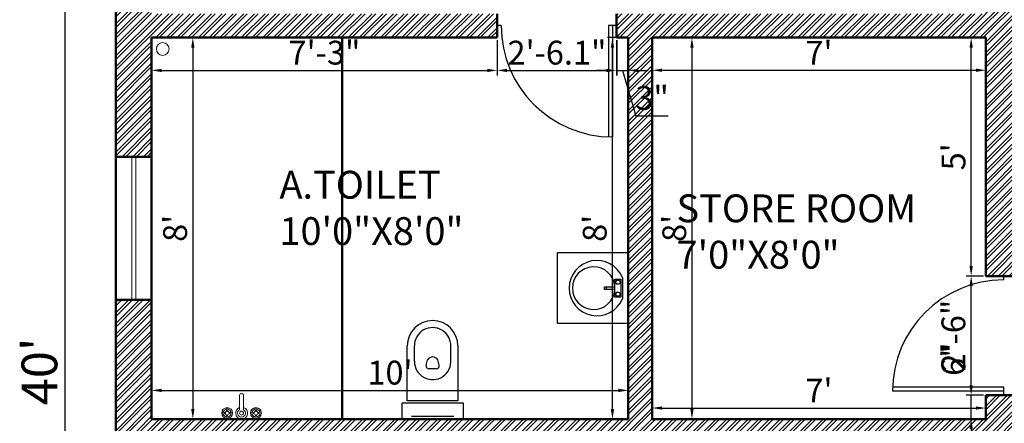
# Model space of a CAD drawing. Units: inches. Extents: x 3590 to 5167, y 65 to 1917.
# Tile 9 of 100: x 4396 to 4644, y 336 to 438. Entities that reach past the tile are written whole.
import ezdxf

# ---------------------------------------------------------------- set-up
doc = ezdxf.new("R2010")
doc.units = ezdxf.units.IN
for name, color, linetype, lineweight in [('A-ANNO-DIMS', 2, 'Continuous', 18), ('A-AREA-IDEN', 7, 'Continuous', 18), ('A-DOOR', 3, 'Continuous', 25), ('A-FLOR-FIXT', 8, 'Continuous', 18), ('A-GLAZ', 4, 'Continuous', 18), ('A-WALL', 7, 'Continuous', 50), ('A-WALL-PATT', 251, 'Continuous', 13)]:
    doc.layers.add(name, color=color, linetype=linetype, lineweight=lineweight)
doc.layers.add('SANTEH', color=7, linetype='Continuous')
doc.styles.get("Standard").update_dxf_attribs({"font": 'arial.ttf'})
doc.dimstyles.new('ISO-25', dxfattribs={"dimtxt": 9, "dimasz": 2.5, "dimexe": 1.25, "dimexo": 0.625, "dimtad": 1, "dimdec": 1, "dimlunit": 3, "dimtxsty": 'Standard', "dimcen": 2.5, "dimadec": 0, "dimazin": 0, "dimtfac": 1, "dimtdec": 1, "dimtmove": 0, "dimatfit": 3, "dimfxl": 1, "dimarcsym": 0})

# ---------------------------------------------------------------- blocks, each defined once
blk = doc.blocks.new('*D280')
at = {"layer": 'A-ANNO-DIMS', "color": 0, "lineweight": -2, "transparency": 16777216}
for p, q in [((4419.65, 589.06), (4406.15, 589.06)), ((4407.4, 586.56), (4407.4, 111.56)), ((4419.65, 109.06), (4406.15, 109.06))]:
    blk.add_line(p, q, dxfattribs=at)
at = {"layer": 'A-ANNO-DIMS', "color": 0, "transparency": 16777216}
for points in [[(4406.98, 586.56), (4407.82, 586.56), (4407.4, 589.06)], [(4406.98, 111.56), (4407.82, 111.56), (4407.4, 109.06)]]:
    blk.add_solid(points, dxfattribs=at)
at = {"layer": 'Defpoints', "color": 0, "transparency": 16777216}
for p in [(4420.27, 589.06), (4407.4, 109.06), (4420.27, 109.06)]:
    blk.add_point(p, dxfattribs=at)
at = {"layer": 'A-ANNO-DIMS', "color": 0, "transparency": 16777216, "insert": (4402.18, 349.06), "char_height": 9, "attachment_point": 5, "rotation": 90}
blk.add_mtext("40'", dxfattribs=at)
blk = doc.blocks.new('D2')
for p, q in [((1, 0), (1, 28)), ((2, 0), (2, 27.98)), ((0, 0), (2, 0)), ((29, 0), (30, 0))]:
    blk.add_line(p, q)
at = {"ltscale": 0.5}
blk.add_arc((1, 0), 28, 0, 90, dxfattribs=at)
blk = doc.blocks.new('*D270')
at = {"layer": 'A-ANNO-DIMS', "color": 0, "lineweight": -2, "transparency": 16777216}
for p, q in [((4429.9, 433.06), (4440.89, 433.06)), ((4439.64, 430.56), (4439.64, 339.56)), ((4429.9, 337.06), (4440.89, 337.06))]:
    blk.add_line(p, q, dxfattribs=at)
at = {"layer": 'A-ANNO-DIMS', "color": 0, "transparency": 16777216}
for points in [[(4439.22, 430.56), (4440.05, 430.56), (4439.64, 433.06)], [(4439.22, 339.56), (4440.05, 339.56), (4439.64, 337.06)]]:
    blk.add_solid(points, dxfattribs=at)
at = {"layer": 'Defpoints', "color": 0, "transparency": 16777216}
for p in [(4429.27, 433.06), (4429.27, 337.06), (4439.64, 337.06)]:
    blk.add_point(p, dxfattribs=at)
at = {"layer": 'A-ANNO-DIMS', "color": 0, "transparency": 16777216, "insert": (4435.95, 385.06), "char_height": 6, "attachment_point": 5, "rotation": 90}
blk.add_mtext("8'", dxfattribs=at)
blk = doc.blocks.new('*D271')
at = {"layer": 'A-ANNO-DIMS', "color": 0, "lineweight": -2, "transparency": 16777216}
for p, q in [((4429.27, 337.68), (4429.27, 345.53)), ((4549.27, 337.68), (4549.27, 345.53)), ((4431.77, 344.28), (4546.77, 344.28))]:
    blk.add_line(p, q, dxfattribs=at)
at = {"layer": 'A-ANNO-DIMS', "color": 0, "transparency": 16777216}
for points in [[(4431.77, 344.7), (4431.77, 343.86), (4429.27, 344.28)], [(4546.77, 344.7), (4546.77, 343.86), (4549.27, 344.28)]]:
    blk.add_solid(points, dxfattribs=at)
at = {"layer": 'Defpoints', "color": 0, "transparency": 16777216}
for p in [(4549.27, 344.28), (4429.27, 337.06), (4549.27, 337.06)]:
    blk.add_point(p, dxfattribs=at)
at = {"layer": 'A-ANNO-DIMS', "color": 0, "transparency": 16777216, "insert": (4489.27, 347.97), "char_height": 6, "attachment_point": 5}
blk.add_mtext("10'", dxfattribs=at)
blk = doc.blocks.new('*D272')
at = {"layer": 'A-ANNO-DIMS', "color": 0, "lineweight": -2, "transparency": 16777216}
for p, q in [((4548.65, 433.06), (4544.02, 433.06)), ((4545.27, 339.56), (4545.27, 430.56)), ((4548.65, 337.06), (4544.02, 337.06))]:
    blk.add_line(p, q, dxfattribs=at)
at = {"layer": 'A-ANNO-DIMS', "color": 0, "transparency": 16777216}
for points in [[(4544.86, 430.56), (4545.69, 430.56), (4545.27, 433.06)], [(4544.86, 339.56), (4545.69, 339.56), (4545.27, 337.06)]]:
    blk.add_solid(points, dxfattribs=at)
at = {"layer": 'Defpoints', "color": 0, "transparency": 16777216}
for p in [(4545.27, 433.06), (4549.27, 433.06), (4549.27, 337.06)]:
    blk.add_point(p, dxfattribs=at)
at = {"layer": 'A-ANNO-DIMS', "color": 0, "transparency": 16777216, "insert": (4541.59, 385.06), "char_height": 6, "attachment_point": 5, "rotation": 90}
blk.add_mtext("8'", dxfattribs=at)
blk = doc.blocks.new('*D273')
at = {"layer": 'A-ANNO-DIMS', "color": 0, "lineweight": -2, "transparency": 16777216}
for p, q in [((4429.27, 432.43), (4429.27, 423.55)), ((4516.27, 432.43), (4516.27, 423.55)), ((4431.77, 424.8), (4513.77, 424.8))]:
    blk.add_line(p, q, dxfattribs=at)
at = {"layer": 'A-ANNO-DIMS', "color": 0, "transparency": 16777216}
for points in [[(4431.77, 425.21), (4431.77, 424.38), (4429.27, 424.8)], [(4513.77, 425.21), (4513.77, 424.38), (4516.27, 424.8)]]:
    blk.add_solid(points, dxfattribs=at)
at = {"layer": 'Defpoints', "color": 0, "transparency": 16777216}
for p in [(4429.27, 433.06), (4516.27, 433.06), (4516.27, 424.8)]:
    blk.add_point(p, dxfattribs=at)
at = {"layer": 'A-ANNO-DIMS', "color": 0, "transparency": 16777216, "insert": (4472.77, 428.49), "char_height": 6, "attachment_point": 5}
blk.add_mtext('7\'-3"', dxfattribs=at)
blk = doc.blocks.new('*D266')
at = {"layer": 'A-ANNO-DIMS', "color": 0, "lineweight": -2, "transparency": 16777216}
for p, q in [((4516.27, 432.43), (4516.27, 423.55)), ((4546.34, 432.43), (4546.34, 423.55)), ((4518.77, 424.8), (4543.84, 424.8))]:
    blk.add_line(p, q, dxfattribs=at)
at = {"layer": 'A-ANNO-DIMS', "color": 0, "transparency": 16777216}
for points in [[(4518.77, 425.21), (4518.77, 424.38), (4516.27, 424.8)], [(4543.84, 425.21), (4543.84, 424.38), (4546.34, 424.8)]]:
    blk.add_solid(points, dxfattribs=at)
at = {"layer": 'Defpoints', "color": 0, "transparency": 16777216}
for p in [(4516.27, 433.06), (4546.34, 433.06), (4546.34, 424.8)]:
    blk.add_point(p, dxfattribs=at)
at = {"layer": 'A-ANNO-DIMS', "color": 0, "transparency": 16777216, "insert": (4531.31, 428.49), "char_height": 6, "attachment_point": 5}
blk.add_mtext('2\'-6.1"', dxfattribs=at)
blk = doc.blocks.new('*D167')
at = {"layer": 'A-ANNO-DIMS', "color": 0, "lineweight": -2, "transparency": 16777216}
for p, q in [((4546.27, 432.43), (4546.27, 423.55)), ((4549.27, 432.43), (4549.27, 423.55)), ((4543.77, 424.8), (4541.27, 424.8)), ((4546.27, 424.8), (4549.27, 424.8)), ((4546.27, 424.8), (4549.27, 424.8)), ((4547.77, 424.8), (4551.19, 413.41)), ((4551.77, 424.8), (4554.27, 424.8)), ((4551.19, 413.41), (4559.33, 413.41))]:
    blk.add_line(p, q, dxfattribs=at)
at = {"layer": 'A-ANNO-DIMS', "color": 0, "transparency": 16777216}
for points in [[(4543.77, 425.21), (4543.77, 424.38), (4546.27, 424.8)], [(4551.77, 425.21), (4551.77, 424.38), (4549.27, 424.8)]]:
    blk.add_solid(points, dxfattribs=at)
at = {"layer": 'Defpoints', "color": 0, "transparency": 16777216}
for p in [(4546.27, 433.06), (4549.27, 433.06), (4549.27, 424.8)]:
    blk.add_point(p, dxfattribs=at)
at = {"layer": 'A-ANNO-DIMS', "color": 0, "transparency": 16777216, "insert": (4555.26, 417.1), "char_height": 6, "attachment_point": 5}
blk.add_mtext('3"', dxfattribs=at)
blk = doc.blocks.new('*D267')
at = {"layer": 'A-ANNO-DIMS', "color": 0, "lineweight": -2, "transparency": 16777216}
for p, q in [((4555.27, 432.43), (4555.27, 423.59)), ((4639.27, 432.43), (4639.27, 423.59)), ((4557.77, 424.84), (4636.77, 424.84))]:
    blk.add_line(p, q, dxfattribs=at)
at = {"layer": 'A-ANNO-DIMS', "color": 0, "transparency": 16777216}
for points in [[(4557.77, 425.25), (4557.77, 424.42), (4555.27, 424.84)], [(4636.77, 425.25), (4636.77, 424.42), (4639.27, 424.84)]]:
    blk.add_solid(points, dxfattribs=at)
at = {"layer": 'Defpoints', "color": 0, "transparency": 16777216}
for p in [(4555.27, 433.06), (4639.27, 433.06), (4639.27, 424.84)]:
    blk.add_point(p, dxfattribs=at)
at = {"layer": 'A-ANNO-DIMS', "color": 0, "transparency": 16777216, "insert": (4597.27, 428.46), "char_height": 6, "attachment_point": 5}
blk.add_mtext("7'", dxfattribs=at)
blk = doc.blocks.new('*D268')
at = {"layer": 'A-ANNO-DIMS', "color": 0, "lineweight": -2, "transparency": 16777216}
for p, q in [((4555.9, 433.06), (4566.54, 433.06)), ((4565.29, 430.56), (4565.29, 339.56)), ((4555.9, 337.06), (4566.54, 337.06))]:
    blk.add_line(p, q, dxfattribs=at)
at = {"layer": 'A-ANNO-DIMS', "color": 0, "transparency": 16777216}
for points in [[(4564.88, 430.56), (4565.71, 430.56), (4565.29, 433.06)], [(4564.88, 339.56), (4565.71, 339.56), (4565.29, 337.06)]]:
    blk.add_solid(points, dxfattribs=at)
at = {"layer": 'Defpoints', "color": 0, "transparency": 16777216}
for p in [(4555.27, 433.06), (4555.27, 337.06), (4565.29, 337.06)]:
    blk.add_point(p, dxfattribs=at)
at = {"layer": 'A-ANNO-DIMS', "color": 0, "transparency": 16777216, "insert": (4561.61, 385.06), "char_height": 6, "attachment_point": 5, "rotation": 90}
blk.add_mtext("8'", dxfattribs=at)
blk = doc.blocks.new('*D261')
at = {"layer": 'A-ANNO-DIMS', "color": 0, "lineweight": -2, "transparency": 16777216}
for p, q in [((4555.27, 337.68), (4555.27, 341.09)), ((4557.77, 339.84), (4636.77, 339.84)), ((4639.27, 337.68), (4639.27, 341.09))]:
    blk.add_line(p, q, dxfattribs=at)
at = {"layer": 'A-ANNO-DIMS', "color": 0, "transparency": 16777216}
for points in [[(4557.77, 340.25), (4557.77, 339.42), (4555.27, 339.84)], [(4636.77, 340.25), (4636.77, 339.42), (4639.27, 339.84)]]:
    blk.add_solid(points, dxfattribs=at)
at = {"layer": 'Defpoints', "color": 0, "transparency": 16777216}
for p in [(4639.27, 339.84), (4555.27, 337.06), (4639.27, 337.06)]:
    blk.add_point(p, dxfattribs=at)
at = {"layer": 'A-ANNO-DIMS', "color": 0, "transparency": 16777216, "insert": (4597.27, 343.46), "char_height": 6, "attachment_point": 5}
blk.add_mtext("7'", dxfattribs=at)
blk = doc.blocks.new('*D262')
at = {"layer": 'A-ANNO-DIMS', "color": 0, "lineweight": -2, "transparency": 16777216}
for p, q in [((4635.58, 345.56), (4635.58, 356.24)), ((4638.65, 343.06), (4634.33, 343.06)), ((4635.58, 337.06), (4635.58, 343.06)), ((4638.65, 337.06), (4634.33, 337.06)), ((4635.58, 334.56), (4635.58, 332.06))]:
    blk.add_line(p, q, dxfattribs=at)
at = {"layer": 'A-ANNO-DIMS', "color": 0, "transparency": 16777216}
for points in [[(4635.17, 345.56), (4636, 345.56), (4635.58, 343.06)], [(4635.17, 334.56), (4636, 334.56), (4635.58, 337.06)]]:
    blk.add_solid(points, dxfattribs=at)
at = {"layer": 'Defpoints', "color": 0, "transparency": 16777216}
for p in [(4635.58, 343.06), (4639.27, 343.06), (4639.27, 337.06)]:
    blk.add_point(p, dxfattribs=at)
at = {"layer": 'A-ANNO-DIMS', "color": 0, "transparency": 16777216, "insert": (4631.89, 352.15), "char_height": 6, "attachment_point": 5, "rotation": 90}
blk.add_mtext('6"', dxfattribs=at)
blk = doc.blocks.new('*D263')
at = {"layer": 'A-ANNO-DIMS', "color": 0, "lineweight": -2, "transparency": 16777216}
for p, q in [((4638.65, 373.06), (4634.33, 373.06)), ((4635.58, 345.56), (4635.58, 370.56)), ((4638.65, 343.06), (4634.33, 343.06))]:
    blk.add_line(p, q, dxfattribs=at)
at = {"layer": 'A-ANNO-DIMS', "color": 0, "transparency": 16777216}
for points in [[(4635.17, 370.56), (4636, 370.56), (4635.58, 373.06)], [(4635.17, 345.56), (4636, 345.56), (4635.58, 343.06)]]:
    blk.add_solid(points, dxfattribs=at)
at = {"layer": 'Defpoints', "color": 0, "transparency": 16777216}
for p in [(4635.58, 373.06), (4639.27, 373.06), (4639.27, 343.06)]:
    blk.add_point(p, dxfattribs=at)
at = {"layer": 'A-ANNO-DIMS', "color": 0, "transparency": 16777216, "insert": (4631.89, 358.06), "char_height": 6, "attachment_point": 5, "rotation": 90}
blk.add_mtext('2\'-6"', dxfattribs=at)
blk = doc.blocks.new('*D264')
at = {"layer": 'A-ANNO-DIMS', "color": 0, "lineweight": -2, "transparency": 16777216}
for p, q in [((4638.65, 433.06), (4634.33, 433.06)), ((4635.58, 375.56), (4635.58, 430.56)), ((4638.65, 373.06), (4634.33, 373.06))]:
    blk.add_line(p, q, dxfattribs=at)
at = {"layer": 'A-ANNO-DIMS', "color": 0, "transparency": 16777216}
for points in [[(4635.17, 430.56), (4636, 430.56), (4635.58, 433.06)], [(4635.17, 375.56), (4636, 375.56), (4635.58, 373.06)]]:
    blk.add_solid(points, dxfattribs=at)
at = {"layer": 'Defpoints', "color": 0, "transparency": 16777216}
for p in [(4635.58, 433.06), (4639.27, 433.06), (4639.27, 373.06)]:
    blk.add_point(p, dxfattribs=at)
at = {"layer": 'A-ANNO-DIMS', "color": 0, "transparency": 16777216, "insert": (4631.91, 403.06), "char_height": 6, "attachment_point": 5, "rotation": 90}
blk.add_mtext("5'", dxfattribs=at)
blk = doc.blocks.new('Faucet - Bathroom top')
for p, q in [((-4.107, 0.125), (-4.375, 0.125)), ((-3.75, 0.4788), (-3.75, 0.75)), ((-3.5, 0.482), (-3.5, 0.75)), ((-3.1461, 0.125), (-2.875, 0.125)), ((3.143, 0.125), (2.875, 0.125)), ((3.5, 0.4788), (3.5, 0.75)), ((3.75, 0.482), (3.75, 0.75)), ((4.1039, 0.125), (4.375, 0.125)), ((-4.1039, -0.125), (-4.375, -0.125)), ((-3.75, -0.4821), (-3.75, -0.75)), ((-3.5, -0.4789), (-3.5, -0.75)), ((-3.143, -0.125), (-2.875, -0.125)), ((-0.5, -0.8639), (-0.5, -4.5)), ((0.5, -4.5), (0.5, -0.8631)), ((3.1461, -0.125), (2.875, -0.125)), ((3.5, -0.4821), (3.5, -0.75)), ((3.75, -0.4789), (3.75, -0.75)), ((4.107, -0.125), (4.375, -0.125))]:
    blk.add_line(p, q)
for centre, radius in [((-3.625, 0), 1.375), ((-4.625, 0), 0.2795), ((-3.625, 0), 0.5), ((-3.625, 1), 0.2795), ((-2.625, 0), 0.2795), ((0, 0), 0.5), ((3.625, 0), 1.375), ((2.625, 0), 0.2795), ((3.625, 0), 0.5), ((3.625, 1), 0.2795), ((4.625, 0), 0.2795), ((-3.625, -1), 0.2795), ((3.625, -1), 0.2795)]:
    blk.add_circle(centre, radius)
for centre, radius, start, end in [((-3.625, 0), 1, 105.2407, 164.2093), ((-3.625, 0), 1, 16.44125, 74.07887), ((0, 0), 1.5, 289.6514, 250.3603), ((0, 0), 1, 300.3431, 239.7554), ((3.625, 0), 1, 106.12, 164.0884), ((3.625, 0), 1, 16.23422, 73.90469), ((-3.625, 0), 1, 196.2342, 253.9047), ((-3.625, 0), 1, 286.12, 344.0884), ((3.625, 0), 1, 196.4413, 254.0789), ((3.625, 0), 1, 285.2407, 344.2093), ((0, -4.5), 0.5, 180, 0)]:
    blk.add_arc(centre, radius, start, end)
blk = doc.blocks.new('y3')
at = {"layer": 'SANTEH', "ltscale": 5}
for p, q in [((37.5, 130.7), (37.5, 520.7)), ((87.5, 410.7), (87.5, 520.7)), ((346.6, 426.1), (347.5, 520.7)), ((397.5, 520.7), (397.5, 130.7)), ((171.9, 384.5), (181.1, 421.3)), ((263.1, 384.5), (253.9, 421.3)), ((244.3, 357.8), (190.7, 357.8)), ((397.5, 130.7), (37.5, 130.7)), ((67.5, 20.7), (367.5, 20.7))]:
    blk.add_line(p, q, dxfattribs=at)
blk.add_lwpolyline([(0, 115), (435, 115), (435, 0), (0, 0), (0, 115)], dxfattribs=at)
for centre, radius, start, end in [((217.5, 520.7), 180, 0, 180), ((217.5, 520.7), 130, 359.15795, 180), ((217.5, 410.7), 130, 180, 5.98548), ((217.5, 399.9), 42.2, 30.52342, 149.47658), ((190.7, 377.8), 20, 160.50385, 270), ((244.3, 377.8), 20, 270, 19.49615)]:
    blk.add_arc(centre, radius, start, end, dxfattribs=at)
blk = doc.blocks.new('r11')
at = {"layer": 'SANTEH', "ltscale": 5}
for p, q in [((0, 0), (600, 0)), ((0, -600), (0, 0)), ((600, 0), (600, -600)), ((210.5, -50), (389.5, -50)), ((210.5, -50), (210.5, -50)), ((223.8, -63.2), (376.2, -63.2)), ((223.8, -113.2), (223.8, -63.2)), ((232.7, -78.7), (249.2, -69.1)), ((232.7, -97.7), (232.7, -78.7)), ((249.2, -69.1), (265.7, -78.7)), ((265.7, -78.7), (265.7, -97.7)), ((334.3, -78.7), (350.8, -69.1)), ((334.3, -97.7), (334.3, -78.7)), ((350.8, -69.1), (367.3, -78.7)), ((367.3, -78.7), (367.3, -97.7)), ((376.2, -63.2), (376.2, -113.2)), ((376.2, -113.2), (223.8, -113.2)), ((249.2, -107.2), (232.7, -97.7)), ((265.7, -97.7), (249.2, -107.2)), ((288, -201.6), (288, -113.2)), ((312, -113.2), (312, -201.6)), ((350.8, -107.2), (334.3, -97.7)), ((367.3, -97.7), (350.8, -107.2)), ((312, -184.3), (288, -184.3)), ((312, -201.6), (288, -201.6)), ((600, -600), (0, -600))]:
    blk.add_line(p, q, dxfattribs=at)
for centre, radius, start, end in [((300, -266.2), 234, 112.50001, 67.49999), ((300, -293), 180.2, 93.8183, 86.1817)]:
    blk.add_arc(centre, radius, start, end, dxfattribs=at)

msp = doc.modelspace()

# ---------------------------------------------------------------- hatches: boundary and pattern name
at = {"layer": 'A-WALL-PATT', "transparency": 33554687}
h = msp.add_hatch(dxfattribs=at)
h.set_pattern_fill('ANSI32', color=256, scale=0.2)
h.set_pattern_definition([(45, (0, -1216.9392), (-1.3470384, 1.3470384), []), (45, (0.898, -1216.9392), (-1.3470384, 1.3470384), [])])
h.paths.add_polyline_path([(4684.27, 589.06), (4591.27, 589.06), (4591.27, 580.06), (4639.27, 580.06), (4639.27, 574.06), (4648.27, 574.06), (4648.27, 580.06), (4684.27, 580.06)])
h.paths.add_polyline_path([(4543.27, 589.06), (4420.27, 589.06), (4420.27, 568.06), (4429.27, 568.06), (4429.27, 580.06), (4445.92, 580.06), (4543.27, 580.06)])
h.paths.add_polyline_path([(4828.27, 589.06), (4744.27, 589.06), (4744.27, 580.06), (4828.27, 580.06)])
h.paths.add_polyline_path([(4648.27, 538.06), (4639.27, 538.06), (4639.27, 439.06), (4546.27, 439.06), (4546.27, 433.06), (4549.27, 433.06), (4549.27, 337.06), (4429.27, 337.06), (4429.27, 367.06), (4420.27, 367.06), (4420.27, 322.06), (4429.27, 322.06), (4429.27, 328.06), (4639.27, 328.06), (4639.27, 322.06), (4648.27, 322.06), (4648.27, 343.06), (4639.27, 343.06), (4639.27, 337.06), (4555.27, 337.06), (4555.27, 433.06), (4639.27, 433.06), (4639.27, 373.06), (4648.27, 373.06)])
h.paths.add_polyline_path([(4516.27, 439.06), (4429.27, 439.06), (4429.27, 520.06), (4420.27, 520.06), (4420.27, 403.06), (4429.27, 403.06), (4429.27, 433.06), (4516.27, 433.06)], flags=17)
h.paths.add_polyline_path([(5080.27, 589.06), (4888.27, 589.06), (4888.27, 580.06), (4924.27, 580.06), (4924.27, 538.06), (4933.27, 538.06), (4933.27, 580.06), (5071.27, 580.06), (5071.27, 118.06), (4933.27, 118.06), (4933.27, 349.06), (4924.27, 349.06), (4924.27, 118.06), (4898.77, 118.06), (4898.77, 109.06), (5080.27, 109.06)])
h.paths.add_polyline_path([(4933.27, 502.06), (4924.27, 502.06), (4924.27, 421.06), (4933.27, 421.06)], flags=17)
h.paths.add_polyline_path([(4802.77, 118.06), (4777.27, 118.06), (4777.27, 286.06), (4756.27, 286.06), (4756.27, 277.06), (4768.27, 277.06), (4768.27, 214.06), (4696.27, 214.06), (4696.27, 277.06), (4708.27, 277.06), (4708.27, 286.06), (4639.27, 286.06), (4639.27, 277.06), (4687.27, 277.06), (4687.27, 214.06), (4681.27, 214.06), (4681.27, 205.06), (4768.27, 205.06), (4768.27, 118.06), (4726.27, 118.06), (4726.27, 109.06), (4802.77, 109.06)])
h.paths.add_polyline_path([(4690.27, 118.06), (4648.27, 118.06), (4648.27, 135.93), (4648.27, 205.06), (4651.27, 205.06), (4651.27, 214.06), (4639.27, 214.06), (4639.27, 118.06), (4633.27, 118.06), (4633.27, 109.06), (4690.27, 109.06)])
h.paths.add_polyline_path([(4585.27, 118.06), (4584.72, 118.06), (4429.27, 118.06), (4429.27, 274.06), (4420.27, 274.06), (4420.27, 109.06), (4585.27, 109.06)])

# ---------------------------------------------------------------- linework, layer by layer
at = {"layer": 'A-FLOR-FIXT'}
msp.add_circle((4432.07, 430.19), 1.6, dxfattribs=at)
at = {"layer": 'A-GLAZ'}
for p, q in [((4424.27, 367.06), (4424.27, 403.06)), ((4425.27, 367.06), (4425.27, 403.06))]:
    msp.add_line(p, q, dxfattribs=at)
at = {"layer": 'A-WALL'}
for p, q in [((4516.27, 433.06), (4516.27, 439.06)), ((4546.27, 433.06), (4546.27, 439.06)), ((4429.27, 433.06), (4516.27, 433.06)), ((4429.27, 337.06), (4429.27, 433.06)), ((4477.27, 337.06), (4477.27, 433.06)), ((4546.27, 433.06), (4549.27, 433.06)), ((4549.27, 337.06), (4549.27, 433.06)), ((4555.27, 433.06), (4639.27, 433.06)), ((4555.27, 337.06), (4555.27, 433.06)), ((4639.27, 373.06), (4639.27, 433.06)), ((4429.27, 403.06), (4420.27, 403.06)), ((4648.27, 373.06), (4639.27, 373.06)), ((4429.27, 367.06), (4420.27, 367.06)), ((4648.27, 343.06), (4639.27, 343.06)), ((4639.27, 337.06), (4639.27, 343.06)), ((4549.27, 337.06), (4429.27, 337.06)), ((4639.27, 337.06), (4555.27, 337.06))]:
    msp.add_line(p, q, dxfattribs=at)
msp.add_lwpolyline([(5080.27, 589.06), (5080.27, 109.06), (4420.27, 109.06), (4420.27, 589.06)], close=True, dxfattribs=at)

# ---------------------------------------------------------------- block references
at = {"layer": 'A-DOOR'}
for p, rotation in [((4546.27, 436.06), 180), ((4643.77, 343.06), 89.99999999999999)]:
    msp.add_blockref('D2', p, dxfattribs=dict(at, rotation=rotation))
at = {"layer": 'A-FLOR-FIXT', "xscale": 0.0297800069284724, "yscale": 0.0297800069284724, "zscale": 0.0297800069284724, "rotation": 270}
msp.add_blockref('r11', (4549.27, 378.94), dxfattribs=at)
at = {"layer": 'A-FLOR-FIXT', "xscale": 0.0353848906415677, "yscale": 0.0353848906415677, "zscale": 0.0353848906415677}
msp.add_blockref('y3', (4492.31, 337.06), dxfattribs=at)
at = {"layer": 'A-FLOR-FIXT', "xscale": -1, "rotation": 180}
msp.add_blockref('Faucet - Bathroom top', (4451.9, 338.56), dxfattribs=at)

# ---------------------------------------------------------------- texts
at = {"layer": 'A-AREA-IDEN', "char_height": 7, "attachment_point": 1}
for s, width, insert in [('{\\fTimes New Roman|b0|i0|c0|p18;A.TOILET\\P10\'0"X8\'0"}', 67.3508, (4461.44, 399.53)), ('{\\fTimes New Roman|b0|i0|c0|p18;STORE ROOM\\P7\'0"X8\'0"}', 98.6883, (4561.41, 393.59))]:
    msp.add_mtext_dynamic_manual_height_columns(s, width=width, gutter_width=12.5, heights=[0], dxfattribs=dict(at, insert=insert))

# ---------------------------------------------------------------- dimensions: what is measured, and where the dimension line sits
at = {"layer": 'A-ANNO-DIMS'}
for base, p1, p2, override, picture, middle in [((4407.4, 109.06), (4420.27, 589.06), (4420.27, 109.06), {"dimclrd": 0, "dimclre": 0, "dimclrt": 0}, '*D280', (4402.18, 349.06)), ((4439.64, 337.06), (4429.27, 433.06), (4429.27, 337.06), {"dimtxt": 6, "dimclrd": 0, "dimclre": 0, "dimclrt": 0}, '*D270', (4435.95, 385.06)), ((4545.27, 433.06), (4549.27, 337.06), (4549.27, 433.06), {"dimtxt": 6, "dimclrd": 0, "dimclre": 0, "dimclrt": 0}, '*D272', (4541.59, 385.06)), ((4565.29, 337.06), (4555.27, 433.06), (4555.27, 337.06), {"dimtxt": 6, "dimclrd": 0, "dimclre": 0, "dimclrt": 0}, '*D268', (4561.61, 385.06)), ((4635.58, 433.06), (4639.27, 373.06), (4639.27, 433.06), {"dimtxt": 6, "dimclrd": 0, "dimclre": 0, "dimclrt": 0, "dimtmove": 1}, '*D264', (4631.91, 403.06)), ((4635.58, 373.06), (4639.27, 343.06), (4639.27, 373.06), {"dimtxt": 6, "dimclrd": 0, "dimclre": 0, "dimclrt": 0, "dimtmove": 1}, '*D263', (4631.89, 358.06)), ((4635.58, 343.06), (4639.27, 337.06), (4639.27, 343.06), {"dimtxt": 6, "dimclrd": 0, "dimclre": 0, "dimclrt": 0}, '*D262', (4631.89, 352.15))]:
    dim = msp.add_linear_dim(base=base, p1=p1, p2=p2, angle=90, dimstyle='ISO-25', override=override, dxfattribs=at)
    dim.commit()
    dim.dimension.update_dxf_attribs({"geometry": picture, "text_midpoint": middle})
for base, p1, p2, override, picture, middle in [((4516.27, 424.8), (4429.27, 433.06), (4516.27, 433.06), {"dimtxt": 6, "dimclrd": 0, "dimclre": 0, "dimclrt": 0}, '*D273', (4472.77, 428.49)), ((4546.34, 424.8), (4516.27, 433.06), (4546.34, 433.06), {"dimtxt": 6, "dimclrd": 0, "dimclre": 0, "dimclrt": 0, "dimtmove": 1}, '*D266', (4531.31, 428.49)), ((4549.27, 424.8), (4546.27, 433.06), (4549.27, 433.06), {"dimtxt": 6, "dimclrd": 0, "dimclre": 0, "dimclrt": 0, "dimtmove": 1}, '*D167', (4551.81, 417.1)), ((4639.27, 424.84), (4555.27, 433.06), (4639.27, 433.06), {"dimtxt": 6, "dimclrd": 0, "dimclre": 0, "dimclrt": 0}, '*D267', (4597.27, 428.46)), ((4549.27, 344.28), (4429.27, 337.06), (4549.27, 337.06), {"dimtxt": 6, "dimclrd": 0, "dimclre": 0, "dimclrt": 0}, '*D271', (4489.27, 347.97)), ((4639.27, 339.84), (4555.27, 337.06), (4639.27, 337.06), {"dimtxt": 6, "dimclrd": 0, "dimclre": 0, "dimclrt": 0}, '*D261', (4597.27, 343.46))]:
    dim = msp.add_linear_dim(base=base, p1=p1, p2=p2, dimstyle='ISO-25', override=override, dxfattribs=at)
    dim.commit()
    dim.dimension.update_dxf_attribs({"geometry": picture, "text_midpoint": middle})

doc.saveas('drawing.dxf')
